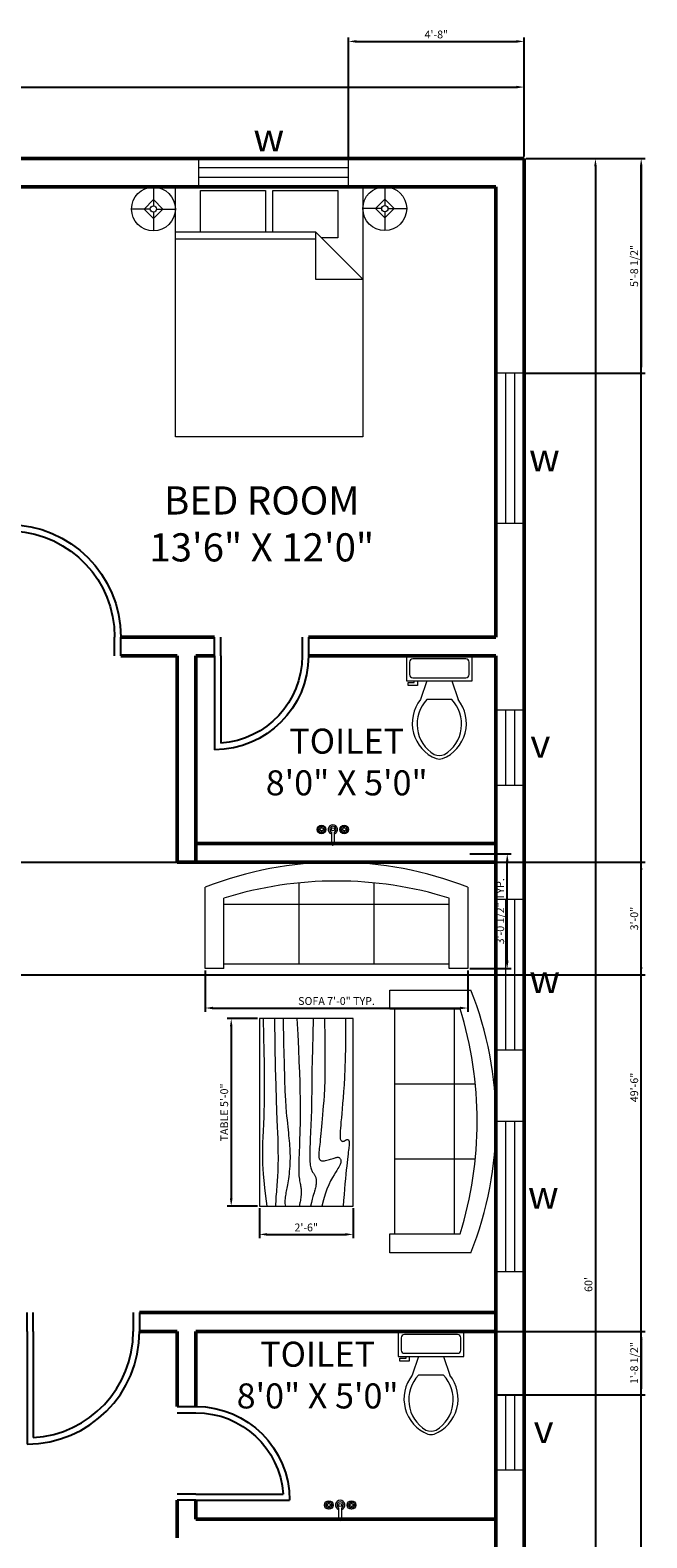
# Model space of a CAD drawing. Units: inches. Extents: x 1776 to 2338, y 1299 to 2099.
# Tile 4 of 4: x 2141 to 2338, y 1617 to 2099. Entities that reach past the tile are written whole.
import ezdxf

# ---------------------------------------------------------------- set-up
doc = ezdxf.new("R2010")
doc.units = ezdxf.units.IN
for name, color, linetype, lineweight in [('A-ANNO-DIMS', 2, 'Continuous', 18), ('A-ANNO-TEXT', 7, 'Continuous', 18), ('A-AREA-IDEN', 7, 'Continuous', 25), ('A-DOOR', 4, 'Continuous', 25), ('A-FLOR-FIXT', 9, 'Continuous', 18), ('A-FURN', 8, 'Continuous', 18), ('A-GLAZ', 4, 'Continuous', 18), ('A-WALL', 7, 'Continuous', 50), ('E-LITE', 9, 'Continuous', 18)]:
    doc.layers.add(name, color=color, linetype=linetype, lineweight=lineweight)
doc.styles.get("Standard").update_dxf_attribs({"font": 'arial.ttf'})
doc.dimstyles.new('ISO-25', dxfattribs={"dimtxt": 2.5, "dimasz": 2.5, "dimexe": 1.25, "dimexo": 0.625, "dimtad": 1, "dimdec": 0, "dimlunit": 3, "dimtxsty": 'Standard', "dimcen": 2.5, "dimadec": 0, "dimazin": 0, "dimtfac": 1, "dimtdec": 0, "dimtmove": 0, "dimatfit": 3, "dimfxl": 1, "dimarcsym": 0})

# ---------------------------------------------------------------- blocks, each defined once
blk = doc.blocks.new('Bed - Queen')
for p, q in [((0, -80.00003), (0, 0)), ((0, 0), (59.99999, 0)), ((59.99999, 0), (59.99999, -80.00003)), ((7.99999, -1.2), (28.79998, -1.2)), ((7.99999, -14.4), (7.99999, -1.2)), ((28.79998, -1.2), (28.79998, -14.4)), ((31.19999, -1.2), (51.99999, -1.2)), ((31.19999, -14.4), (31.19999, -1.2)), ((51.99999, -1.2), (51.99999, -16.4)), ((0, -14.4), (44.8, -14.4)), ((59.99999, -29.6), (44.8, -14.4)), ((44.8, -14.4), (44.8, -29.6)), ((44.8, -16.8), (0, -16.8)), ((51.99999, -16.4), (46.79936, -16.4)), ((44.8, -29.6), (59.99999, -29.6)), ((59.99999, -80.00003), (0, -80.00003))]:
    blk.add_line(p, q)
blk = doc.blocks.new('Sofa - Roundback 7 ft.')
for p, q in [((-12.00002, -32.4421), (-12.00003, -6.5971)), ((11.99997, -32.4421), (11.99998, -6.5971)), ((-36.000027, -34), (-36.000027, -11.4696)), ((-35.999844, -13.3819), (35.9998, -13.3819)), ((35.99998, -34), (35.99998, -11.4696)), ((-36.000027, -32.4421), (35.99998, -32.4421))]:
    blk.add_line(p, q)
for points in [[(-36.000027, -34), (-42.000027, -34), (-42.000027, -8)], [(41.99998, -8), (41.99998, -34), (35.99998, -34)]]:
    blk.add_lwpolyline(points)
for centre, radius, start, end in [((0, -114.25), 114.25, 68.43141, 111.5686), ((-0.00001, -127.1968), 121.1968, 72.72033, 107.2797)]:
    blk.add_arc(centre, radius, start, end)
blk = doc.blocks.new('Table - Rectangular Woodgrain 60 x 30 in.')
for p, q in [((0, 0), (0, -30)), ((60, 0), (0, 0)), ((60, -30), (60, 0)), ((0, -30), (60, -30))]:
    blk.add_line(p, q)
for points in [[(0, -2.4), (4.8155, -2.418), (9.0302, -2.4688), (12.709, -2.5477), (15.9167, -2.65), (18.7181, -2.7711), (21.1781, -2.9063), (23.3616, -3.0508), (25.3333, -3.2), (27.1477, -3.3495), (28.8172, -3.4958), (30.3437, -3.636), (31.7291, -3.7667), (32.9756, -3.8849), (34.0849, -3.9875), (35.059, -4.0714), (35.9, -4.1334), (36.6114, -4.1711), (37.2041, -4.1854), (37.6906, -4.1779), (38.0833, -4.15), (38.3948, -4.1034), (38.6375, -4.0396), (38.8239, -3.9602), (38.9666, -3.8667), (39.0764, -3.7608), (39.1573, -3.6448), (39.2116, -3.521), (39.2416, -3.3917), (39.2498, -3.2593), (39.2385, -3.1261), (39.21, -2.9944), (39.1666, -2.8667), (39.111, -2.7447), (39.0468, -2.6281), (38.978, -2.5163), (38.9083, -2.4083), (38.8418, -2.3035), (38.7823, -2.201), (38.7337, -2.1001), (38.7, -2), (38.6844, -1.9003), (38.6875, -1.8021), (38.7094, -1.707), (38.75, -1.6167), (38.8094, -1.5326), (38.8875, -1.4563), (38.9844, -1.3893), (39.1, -1.3333), (39.2351, -1.2896), (39.3937, -1.2583), (39.5804, -1.2396), (39.8, -1.2333), (40.057, -1.2396), (40.3562, -1.2583), (40.7023, -1.2896), (41.1, -1.3333), (41.5547, -1.3895), (42.0755, -1.4573), (42.6721, -1.5361), (43.3542, -1.625), (44.1316, -1.7233), (45.014, -1.8302), (46.0114, -1.9449), (47.1333, -2.0667), (48.3862, -2.1947), (49.7625, -2.3281), (51.2513, -2.4663), (52.8416, -2.6083), (54.5226, -2.7535), (56.2833, -2.9011), (58.1127, -3.0501), (60, -3.2)], [(0, -9.2), (6.5759, -9.0858), (11.9385, -9.0365), (16.2527, -9.0418), (19.6833, -9.0917), (22.3952, -9.1759), (24.5531, -9.2844), (26.322, -9.4069), (27.8666, -9.5333), (29.3241, -9.6553), (30.7203, -9.7719), (32.0532, -9.8837), (33.3208, -9.9917), (34.5213, -10.0965), (35.6526, -10.199), (36.7128, -10.2999), (37.7, -10.4), (38.6129, -10.4996), (39.4531, -10.5969), (40.223, -10.6895), (40.925, -10.775), (41.5613, -10.8512), (42.1344, -10.9156), (42.6465, -10.966), (43.1, -11), (43.4976, -11.0158), (43.8437, -11.0136), (44.143, -10.9942), (44.4, -10.9583), (44.6195, -10.9069), (44.8062, -10.8406), (44.9648, -10.7603), (45.1, -10.6667), (45.2155, -10.5598), (45.3114, -10.4365), (45.3871, -10.2929), (45.4416, -10.125), (45.4743, -9.929), (45.4844, -9.7011), (45.4709, -9.4371), (45.4333, -9.1333), (45.3716, -8.7883), (45.2896, -8.4104), (45.1919, -8.0107), (45.0833, -7.6), (44.9685, -7.1893), (44.8521, -6.7896), (44.7388, -6.4117), (44.6333, -6.0667), (44.54, -5.7628), (44.4614, -5.4979), (44.4001, -5.2675), (44.3583, -5.0667), (44.3384, -4.8909), (44.3427, -4.7354), (44.3736, -4.5956), (44.4333, -4.4667), (44.5236, -4.3453), (44.6427, -4.2333), (44.7884, -4.1339), (44.9583, -4.05), (45.1501, -3.9849), (45.3614, -3.9417), (45.59, -3.9234), (45.8333, -3.9333), (46.0915, -3.9749), (46.3734, -4.0531), (46.6906, -4.1736), (47.0542, -4.3417), (47.4756, -4.5629), (47.9661, -4.8427), (48.5372, -5.1866), (49.2, -5.6), (49.9676, -6.0844), (50.8594, -6.625), (51.8965, -7.2031), (53.1, -7.8), (54.491, -8.3969), (56.0906, -8.975), (57.9199, -9.5156), (60, -10)], [(0, -12.8), (5.1847, -12.9322), (9.6213, -13.0323), (13.3963, -13.1059), (16.5958, -13.1583), (19.3063, -13.1952), (21.614, -13.2219), (23.6054, -13.2439), (25.3666, -13.2667), (26.9728, -13.2947), (28.4531, -13.3281), (29.8256, -13.3663), (31.1083, -13.4083), (32.3191, -13.4535), (33.476, -13.501), (34.597, -13.5501), (35.7, -13.6), (36.7984, -13.6497), (37.8875, -13.6979), (38.9578, -13.743), (40, -13.7833), (41.0047, -13.8174), (41.9625, -13.8438), (42.864, -13.8607), (43.7, -13.8667), (44.4631, -13.8604), (45.1552, -13.8417), (45.7801, -13.8104), (46.3416, -13.7667), (46.8439, -13.7104), (47.2906, -13.6417), (47.6858, -13.5604), (48.0333, -13.4667), (48.3375, -13.3608), (48.6042, -13.2448), (48.8396, -13.121), (49.05, -12.9917), (49.2417, -12.8593), (49.4208, -12.7261), (49.5937, -12.5944), (49.7667, -12.4667), (49.9452, -12.3451), (50.1323, -12.2313), (50.3303, -12.1268), (50.5416, -12.0333), (50.7686, -11.9524), (51.0135, -11.8854), (51.2788, -11.8341), (51.5666, -11.8), (51.8785, -11.7843), (52.2116, -11.7865), (52.562, -11.8059), (52.926, -11.8417), (53.2998, -11.8931), (53.6795, -11.9594), (54.0614, -12.0397), (54.4416, -12.1333), (54.8223, -12.2401), (55.2293, -12.3625), (55.6942, -12.5037), (56.2489, -12.6667), (56.9251, -12.8547), (57.7545, -13.0708), (58.7689, -13.3182), (60, -13.6)], [(0, -18), (5.124, -17.7273), (9.6609, -17.5057), (13.6705, -17.3303), (17.2125, -17.1958), (20.3467, -17.0973), (23.1328, -17.0297), (25.6307, -16.9878), (27.9, -16.9667), (29.9928, -16.9617), (31.9302, -16.9703), (33.7254, -16.9907), (35.3917, -17.0208), (36.9423, -17.0588), (38.3906, -17.1026), (39.7499, -17.1503), (41.0333, -17.2), (42.2519, -17.2496), (43.4073, -17.2969), (44.4986, -17.3395), (45.525, -17.375), (46.4858, -17.4012), (47.3802, -17.4156), (48.2074, -17.416), (48.9667, -17.4), (49.6583, -17.3662), (50.2872, -17.3167), (50.8595, -17.2547), (51.3812, -17.1833), (51.8584, -17.1057), (52.2971, -17.025), (52.7034, -16.9443), (53.0833, -16.8667), (53.443, -16.7951), (53.789, -16.7313), (54.128, -16.6768), (54.4666, -16.6334), (54.8115, -16.6024), (55.1693, -16.5854), (55.5465, -16.5841), (55.95, -16.6), (56.3828, -16.6337), (56.8346, -16.6823), (57.2915, -16.7418), (57.7396, -16.8084), (58.165, -16.878), (58.5539, -16.9469), (58.8924, -17.0111), (59.1666, -17.0667), (59.3679, -17.1107), (59.5078, -17.1438), (59.6032, -17.1675), (59.6708, -17.1833), (59.7275, -17.193), (59.7901, -17.1979), (59.8753, -17.1998), (60, -17.2)], [(0, -22.4), (8.0098, -22.2501), (14.4094, -22.1011), (19.4168, -21.9535), (23.25, -21.8083), (26.1269, -21.6663), (28.2656, -21.5281), (29.884, -21.3947), (31.2, -21.2667), (32.3967, -21.1448), (33.5172, -21.0292), (34.5697, -20.9198), (35.5625, -20.8167), (36.5037, -20.7198), (37.4015, -20.6292), (38.2642, -20.5448), (39.1, -20.4667), (39.9164, -20.3951), (40.7187, -20.3313), (41.5117, -20.2768), (42.3, -20.2333), (43.0883, -20.2024), (43.8812, -20.1854), (44.6836, -20.1841), (45.5, -20.2), (46.3328, -20.234), (47.1747, -20.2844), (48.0163, -20.3488), (48.8479, -20.425), (49.66, -20.5106), (50.4429, -20.6031), (51.1872, -20.7004), (51.8833, -20.8), (52.5246, -20.8999), (53.1166, -20.9995), (53.6681, -21.0983), (54.1875, -21.1958), (54.6834, -21.2919), (55.1646, -21.3859), (55.6394, -21.4777), (56.1167, -21.5667), (56.6028, -21.6515), (57.0961, -21.7266), (57.5929, -21.7852), (58.0896, -21.8208), (58.5823, -21.8268), (59.0674, -21.7964), (59.5412, -21.723), (60, -21.6)], [(0, -25.2), (8.6355, -25.0504), (15.7026, -24.9031), (21.4049, -24.7606), (25.9458, -24.625), (29.529, -24.4988), (32.3578, -24.3844), (34.6359, -24.284), (36.5667, -24.2), (38.3213, -24.1341), (39.9417, -24.0854), (41.437, -24.0523), (42.8167, -24.0333), (44.0901, -24.0268), (45.2667, -24.0313), (46.3557, -24.0451), (47.3667, -24.0667), (48.309, -24.0947), (49.1928, -24.1287), (50.0284, -24.168), (50.826, -24.2125), (51.5959, -24.2617), (52.3483, -24.3151), (53.0935, -24.3725), (53.8417, -24.4334), (54.6009, -24.497), (55.3699, -24.561), (56.1454, -24.6226), (56.9239, -24.6792), (57.7021, -24.7279), (58.4764, -24.7662), (59.2435, -24.7911), (60, -24.8)], [(0, -28.8), (5.6867, -28.6681), (10.45, -28.5698), (14.407, -28.5012), (17.675, -28.4584), (20.3711, -28.4374), (22.6125, -28.4344), (24.5164, -28.4455), (26.2, -28.4667), (27.762, -28.4947), (29.2276, -28.5281), (30.6033, -28.5663), (31.8958, -28.6084), (33.1118, -28.6535), (34.2578, -28.7011), (35.3405, -28.7501), (36.3666, -28.8), (37.3443, -28.8497), (38.288, -28.8974), (39.2137, -28.9412), (40.1375, -28.9792), (41.0753, -29.0093), (42.0432, -29.0297), (43.0572, -29.0384), (44.1333, -29.0333), (45.2936, -29.0114), (46.5843, -28.9641), (48.0579, -28.8816), (49.7666, -28.7542), (51.7629, -28.5721), (54.0989, -28.3255), (56.8272, -28.0048), (60, -27.6)]]:
    blk.add_lwpolyline(points)
blk = doc.blocks.new('Lamp - Table')
for p, q in [((0, 7), (0, 1)), ((-1, 0), (-7, 0)), ((0, 3), (-3, 0)), ((-3, 0), (0, -3)), ((3, 0), (0, 3)), ((0, -3), (3, 0)), ((1, 0), (7, 0)), ((0, -1), (0, -7))]:
    blk.add_line(p, q)
for radius in [7, 1]:
    blk.add_circle((0, 0), radius)
blk = doc.blocks.new('Toilet - top')
for p, q in [((9.5, -6), (9.5, -2)), ((-10, -8.5), (-8, -8.5)), ((-10, -9.5), (-10, -8.5)), ((-7, -9.5), (-10, -9.5)), ((-8, -8.5), (-8, -8)), ((-7, -8), (-7, -9.5)), ((-4, -8), (-6, -14)), ((4, -8), (6, -14)), ((4, -14), (-4, -14))]:
    blk.add_line(p, q)
blk.add_lwpolyline([(10.5, -8), (10.5, 0), (-10.5, 0), (-10.5, -8)], close=True)
for points in [[(-9.5, -2), (-9.5, -6)], [(8.5, -1), (-8.5, -1)], [(-8.5, -7), (8.5, -7)]]:
    blk.add_lwpolyline(points)
for centre, radius, start, end in [((-8.62, -1.88), 0.884, 81.8699, 188.1301), ((8.62, -1.88), 0.884, 351.8699, 98.1301), ((-8.62, -6.12), 0.884, 171.8699, 278.1301), ((8.62, -6.12), 0.884, 261.8699, 8.1301), ((3.52, -21.58), 12.17, 141.4691, 247.9714), ((4.2, -21.82), 11.33, 136.3677, 238.9468), ((-3.52, -21.58), 12.17, 292.0284, 38.5307), ((-4.2, -21.82), 11.33, 301.053, 43.6321), ((0, -27.88), 4, 245.7318, 294.2682), ((0, -29), 4, 254.8605, 285.1395)]:
    blk.add_arc(centre, radius, start, end)
blk = doc.blocks.new('Faucet - Bathroom top')
for p, q in [((-4.107, 0.125), (-4.375, 0.125)), ((-3.75, 0.4788), (-3.75, 0.75)), ((-3.5, 0.482), (-3.5, 0.75)), ((-3.1461, 0.125), (-2.875, 0.125)), ((3.143, 0.125), (2.875, 0.125)), ((3.5, 0.4788), (3.5, 0.75)), ((3.75, 0.482), (3.75, 0.75)), ((4.1039, 0.125), (4.375, 0.125)), ((-4.1039, -0.125), (-4.375, -0.125)), ((-3.75, -0.4821), (-3.75, -0.75)), ((-3.5, -0.4789), (-3.5, -0.75)), ((-3.143, -0.125), (-2.875, -0.125)), ((-0.5, -0.8639), (-0.5, -4.5)), ((0.5, -4.5), (0.5, -0.8631)), ((3.1461, -0.125), (2.875, -0.125)), ((3.5, -0.4821), (3.5, -0.75)), ((3.75, -0.4789), (3.75, -0.75)), ((4.107, -0.125), (4.375, -0.125))]:
    blk.add_line(p, q)
for centre, radius in [((-3.625, 0), 1.375), ((-4.625, 0), 0.2795), ((-3.625, 0), 0.5), ((-3.625, 1), 0.2795), ((-2.625, 0), 0.2795), ((0, 0), 0.5), ((3.625, 0), 1.375), ((2.625, 0), 0.2795), ((3.625, 0), 0.5), ((3.625, 1), 0.2795), ((4.625, 0), 0.2795), ((-3.625, -1), 0.2795), ((3.625, -1), 0.2795)]:
    blk.add_circle(centre, radius)
for centre, radius, start, end in [((-3.625, 0), 1, 105.2407, 164.2093), ((-3.625, 0), 1, 16.44125, 74.07887), ((0, 0), 1.5, 289.6514, 250.3603), ((0, 0), 1, 300.3431, 239.7554), ((3.625, 0), 1, 106.12, 164.0884), ((3.625, 0), 1, 16.23422, 73.90469), ((-3.625, 0), 1, 196.2342, 253.9047), ((-3.625, 0), 1, 286.12, 344.0884), ((0, -4.5), 0.5, 180, 0), ((3.625, 0), 1, 196.4413, 254.0789), ((3.625, 0), 1, 285.2407, 344.2093)]:
    blk.add_arc(centre, radius, start, end)
blk = doc.blocks.new('*D12')
at = {"layer": 'A-ANNO-DIMS', "color": 0, "lineweight": -2, "transparency": 16777216}
for p, q in [((1818.74, 2058.84), (1818.74, 2082.32)), ((1821.24, 2081.07), (2296.24, 2081.07)), ((2298.74, 2058.84), (2298.74, 2082.32))]:
    blk.add_line(p, q, dxfattribs=at)
at = {"layer": 'A-ANNO-DIMS', "color": 0, "transparency": 16777216}
for points in [[(1821.24, 2081.49), (1821.24, 2080.65), (1818.74, 2081.07)], [(2296.24, 2081.49), (2296.24, 2080.65), (2298.74, 2081.07)]]:
    blk.add_solid(points, dxfattribs=at)
at = {"layer": 'Defpoints', "color": 0, "transparency": 16777216}
for p in [(2298.74, 2081.07), (1818.74, 2058.22), (2298.74, 2058.22)]:
    blk.add_point(p, dxfattribs=at)
at = {"layer": 'A-ANNO-DIMS', "color": 0, "transparency": 16777216, "insert": (2058.74, 2082.97), "char_height": 2.5, "attachment_point": 5}
blk.add_mtext("40'", dxfattribs=at)
blk = doc.blocks.new('*D13')
at = {"layer": 'A-ANNO-DIMS', "color": 0, "lineweight": -2, "transparency": 16777216}
for p, q in [((2299.36, 2058.22), (2322.8, 2058.22)), ((2321.55, 2055.72), (2321.55, 1340.72)), ((2299.36, 1338.22), (2322.8, 1338.22))]:
    blk.add_line(p, q, dxfattribs=at)
at = {"layer": 'A-ANNO-DIMS', "color": 0, "transparency": 16777216}
for points in [[(2321.14, 2055.72), (2321.97, 2055.72), (2321.55, 2058.22)], [(2321.14, 1340.72), (2321.97, 1340.72), (2321.55, 1338.22)]]:
    blk.add_solid(points, dxfattribs=at)
at = {"layer": 'Defpoints', "color": 0, "transparency": 16777216}
for p in [(2298.74, 2058.22), (2298.74, 1338.22), (2321.55, 1338.22)]:
    blk.add_point(p, dxfattribs=at)
at = {"layer": 'A-ANNO-DIMS', "color": 0, "transparency": 16777216, "insert": (2319.65, 1698.22), "char_height": 2.5, "attachment_point": 5, "rotation": 90}
blk.add_mtext("60'", dxfattribs=at)
blk = doc.blocks.new('WIN-48IN')
for p, q in [((48, 9), (0, 9)), ((0, 9), (0, 0)), ((48, 6), (0, 6)), ((48, 0), (48, 9)), ((0, 3), (48, 3)), ((0, 0), (48, 0))]:
    blk.add_line(p, q)
blk = doc.blocks.new('VENT-24IN')
for p, q in [((9, 24), (0, 24)), ((0, 24), (0, 0)), ((3, 24), (3, 0)), ((6, 0), (6, 24)), ((9, 0), (9, 24)), ((0, 0), (9, 0))]:
    blk.add_line(p, q)
blk = doc.blocks.new('DOOR-36IN')
for p, q in [((34, 6), (34, 39.94)), ((36, 6), (36, 42)), ((0, 0), (0, 6)), ((2, 0), (2, 6)), ((34, 6), (34, 0)), ((36, 6), (36, 0))]:
    blk.add_line(p, q)
for radius, start in [(36, 90), (34, 93.3723)]:
    blk.add_arc((36, 6), radius, start, 180)
blk = doc.blocks.new('DOOR-30IN')
for p, q in [((0, 36), (0, 30)), ((2, 36), (2, 30)), ((28, 30), (28, 36)), ((30, 30), (30, 36)), ((28, 30), (28, 2.07)), ((30, 30), (30, 0))]:
    blk.add_line(p, q)
for radius, end in [(30, 270), (28, 265.904)]:
    blk.add_arc((30, 30), radius, 180, end)
blk = doc.blocks.new('*D34')
at = {"layer": 'A-ANNO-DIMS', "color": 0, "lineweight": -2, "transparency": 16777216}
for p, q in [((2196.74, 1798.59), (2196.74, 1785.37)), ((2280.74, 1798.59), (2280.74, 1785.37)), ((2199.24, 1786.62), (2278.24, 1786.62))]:
    blk.add_line(p, q, dxfattribs=at)
at = {"layer": 'A-ANNO-DIMS', "color": 0, "transparency": 16777216}
for points in [[(2199.24, 1787.04), (2199.24, 1786.2), (2196.74, 1786.62)], [(2278.24, 1787.04), (2278.24, 1786.2), (2280.74, 1786.62)]]:
    blk.add_solid(points, dxfattribs=at)
at = {"layer": 'Defpoints', "color": 0, "transparency": 16777216}
for p in [(2196.74, 1799.22), (2280.74, 1799.22), (2280.74, 1786.62)]:
    blk.add_point(p, dxfattribs=at)
at = {"layer": 'A-ANNO-DIMS', "color": 0, "transparency": 16777216, "insert": (2238.74, 1788.54), "char_height": 2.5, "attachment_point": 5}
blk.add_mtext('SOFA 7\'-0" TYP.', dxfattribs=at)
blk = doc.blocks.new('*D35')
at = {"layer": 'A-ANNO-DIMS', "color": 0, "lineweight": -2, "transparency": 16777216}
for p, q in [((2281.36, 1835.89), (2294.59, 1835.89)), ((2293.34, 1801.72), (2293.34, 1833.39)), ((2281.36, 1799.22), (2294.59, 1799.22))]:
    blk.add_line(p, q, dxfattribs=at)
at = {"layer": 'A-ANNO-DIMS', "color": 0, "transparency": 16777216}
for points in [[(2292.92, 1833.39), (2293.76, 1833.39), (2293.34, 1835.89)], [(2292.92, 1801.72), (2293.76, 1801.72), (2293.34, 1799.22)]]:
    blk.add_solid(points, dxfattribs=at)
at = {"layer": 'Defpoints', "color": 0, "transparency": 16777216}
for p in [(2280.74, 1835.89), (2293.34, 1835.89), (2280.74, 1799.22)]:
    blk.add_point(p, dxfattribs=at)
at = {"layer": 'A-ANNO-DIMS', "color": 0, "transparency": 16777216, "insert": (2291.42, 1817.55), "char_height": 2.5, "attachment_point": 5, "rotation": 90}
blk.add_mtext('3\'-0 1/2" TYP.', dxfattribs=at)
blk = doc.blocks.new('*D36')
at = {"layer": 'A-ANNO-DIMS', "color": 0, "lineweight": -2, "transparency": 16777216}
for p, q in [((2213.43, 1783.24), (2203.8, 1783.24)), ((2205.05, 1780.74), (2205.05, 1725.74)), ((2213.43, 1723.24), (2203.8, 1723.24))]:
    blk.add_line(p, q, dxfattribs=at)
at = {"layer": 'A-ANNO-DIMS', "color": 0, "transparency": 16777216}
for points in [[(2204.64, 1780.74), (2205.47, 1780.74), (2205.05, 1783.24)], [(2204.64, 1725.74), (2205.47, 1725.74), (2205.05, 1723.24)]]:
    blk.add_solid(points, dxfattribs=at)
at = {"layer": 'Defpoints', "color": 0, "transparency": 16777216}
for p in [(2214.05, 1783.24), (2205.05, 1723.24), (2214.05, 1723.24)]:
    blk.add_point(p, dxfattribs=at)
at = {"layer": 'A-ANNO-DIMS', "color": 0, "transparency": 16777216, "insert": (2203.15, 1753.24), "char_height": 2.5, "attachment_point": 5, "rotation": 90}
blk.add_mtext('TABLE 5\'-0"', dxfattribs=at)
blk = doc.blocks.new('*D37')
at = {"layer": 'A-ANNO-DIMS', "color": 0, "lineweight": -2, "transparency": 16777216}
for p, q in [((2214.05, 1722.61), (2214.05, 1712.99)), ((2244.05, 1722.61), (2244.05, 1712.99)), ((2216.55, 1714.24), (2241.55, 1714.24))]:
    blk.add_line(p, q, dxfattribs=at)
at = {"layer": 'A-ANNO-DIMS', "color": 0, "transparency": 16777216}
for points in [[(2216.55, 1714.66), (2216.55, 1713.82), (2214.05, 1714.24)], [(2241.55, 1714.66), (2241.55, 1713.82), (2244.05, 1714.24)]]:
    blk.add_solid(points, dxfattribs=at)
at = {"layer": 'Defpoints', "color": 0, "transparency": 16777216}
for p in [(2214.05, 1723.24), (2244.05, 1723.24), (2244.05, 1714.24)]:
    blk.add_point(p, dxfattribs=at)
at = {"layer": 'A-ANNO-DIMS', "color": 0, "transparency": 16777216, "insert": (2229.05, 1716.14), "char_height": 2.5, "attachment_point": 5}
blk.add_mtext('2\'-6"', dxfattribs=at)
blk = doc.blocks.new('*D42')
at = {"layer": 'A-ANNO-DIMS', "color": 0, "lineweight": -2, "transparency": 16777216}
for p, q in [((2299.36, 2058.22), (2337.44, 2058.22)), ((2336.19, 1466.72), (2336.19, 2055.72)), ((2290.36, 1464.22), (2337.44, 1464.22))]:
    blk.add_line(p, q, dxfattribs=at)
at = {"layer": 'A-ANNO-DIMS', "color": 0, "transparency": 16777216}
for points in [[(2335.77, 2055.72), (2336.61, 2055.72), (2336.19, 2058.22)], [(2335.77, 1466.72), (2336.61, 1466.72), (2336.19, 1464.22)]]:
    blk.add_solid(points, dxfattribs=at)
at = {"layer": 'Defpoints', "color": 0, "transparency": 16777216}
for p in [(2298.74, 2058.22), (2336.19, 2058.22), (2289.74, 1464.22)]:
    blk.add_point(p, dxfattribs=at)
at = {"layer": 'A-ANNO-DIMS', "color": 0, "transparency": 16777216, "insert": (2334.29, 1761.22), "char_height": 2.5, "attachment_point": 5, "rotation": 90}
blk.add_mtext('49\'-6"', dxfattribs=at)
blk = doc.blocks.new('*D48')
at = {"layer": 'A-ANNO-DIMS', "color": 0, "lineweight": -2, "transparency": 16777216}
for p, q in [((1936.36, 1833.22), (2337.44, 1833.22)), ((2336.19, 1799.72), (2336.19, 1830.72)), ((1936.36, 1797.22), (2337.44, 1797.22))]:
    blk.add_line(p, q, dxfattribs=at)
at = {"layer": 'A-ANNO-DIMS', "color": 0, "transparency": 16777216}
for points in [[(2335.77, 1830.72), (2336.61, 1830.72), (2336.19, 1833.22)], [(2335.77, 1799.72), (2336.61, 1799.72), (2336.19, 1797.22)]]:
    blk.add_solid(points, dxfattribs=at)
at = {"layer": 'Defpoints', "color": 0, "transparency": 16777216}
for p in [(1935.74, 1833.22), (2336.19, 1833.22), (1935.74, 1797.22)]:
    blk.add_point(p, dxfattribs=at)
at = {"layer": 'A-ANNO-DIMS', "color": 0, "transparency": 16777216, "insert": (2334.29, 1815.22), "char_height": 2.5, "attachment_point": 5, "rotation": 90}
blk.add_mtext('3\'-0"', dxfattribs=at)
blk = doc.blocks.new('*D52')
at = {"layer": 'A-ANNO-DIMS', "color": 0, "lineweight": -2, "transparency": 16777216}
for p, q in [((2242.6, 2058.84), (2242.6, 2096.92)), ((2245.1, 2095.67), (2296.24, 2095.67)), ((2298.74, 2058.84), (2298.74, 2096.92))]:
    blk.add_line(p, q, dxfattribs=at)
at = {"layer": 'A-ANNO-DIMS', "color": 0, "transparency": 16777216}
for points in [[(2245.1, 2096.09), (2245.1, 2095.25), (2242.6, 2095.67)], [(2296.24, 2096.09), (2296.24, 2095.25), (2298.74, 2095.67)]]:
    blk.add_solid(points, dxfattribs=at)
at = {"layer": 'Defpoints', "color": 0, "transparency": 16777216}
for p in [(2298.74, 2095.67), (2242.6, 2058.22), (2298.74, 2058.22)]:
    blk.add_point(p, dxfattribs=at)
at = {"layer": 'A-ANNO-DIMS', "color": 0, "transparency": 16777216, "insert": (2270.67, 2097.57), "char_height": 2.5, "attachment_point": 5}
blk.add_mtext('4\'-8"', dxfattribs=at)
blk = doc.blocks.new('*D54')
at = {"layer": 'A-ANNO-DIMS', "color": 0, "lineweight": -2, "transparency": 16777216}
for p, q in [((2299.36, 2058.22), (2337.44, 2058.22)), ((2336.19, 2055.72), (2336.19, 1992.09)), ((2299.36, 1989.59), (2337.44, 1989.59))]:
    blk.add_line(p, q, dxfattribs=at)
at = {"layer": 'A-ANNO-DIMS', "color": 0, "transparency": 16777216}
for points in [[(2335.77, 2055.72), (2336.61, 2055.72), (2336.19, 2058.22)], [(2335.77, 1992.09), (2336.61, 1992.09), (2336.19, 1989.59)]]:
    blk.add_solid(points, dxfattribs=at)
at = {"layer": 'Defpoints', "color": 0, "transparency": 16777216}
for p in [(2298.74, 2058.22), (2298.74, 1989.59), (2336.19, 1989.59)]:
    blk.add_point(p, dxfattribs=at)
at = {"layer": 'A-ANNO-DIMS', "color": 0, "transparency": 16777216, "insert": (2334.27, 2023.9), "char_height": 2.5, "attachment_point": 5, "rotation": 90}
blk.add_mtext('5\'-8 1/2"', dxfattribs=at)
blk = doc.blocks.new('*D57')
at = {"layer": 'A-ANNO-DIMS', "color": 0, "lineweight": -2, "transparency": 16777216}
for p, q in [((2290.36, 1683.22), (2337.44, 1683.22)), ((2336.19, 1680.72), (2336.19, 1665.46)), ((2290.36, 1662.96), (2337.44, 1662.96))]:
    blk.add_line(p, q, dxfattribs=at)
at = {"layer": 'A-ANNO-DIMS', "color": 0, "transparency": 16777216}
for points in [[(2335.77, 1680.72), (2336.61, 1680.72), (2336.19, 1683.22)], [(2335.77, 1665.46), (2336.61, 1665.46), (2336.19, 1662.96)]]:
    blk.add_solid(points, dxfattribs=at)
at = {"layer": 'Defpoints', "color": 0, "transparency": 16777216}
for p in [(2289.74, 1683.22), (2289.74, 1662.96), (2336.19, 1662.96)]:
    blk.add_point(p, dxfattribs=at)
at = {"layer": 'A-ANNO-DIMS', "color": 0, "transparency": 16777216, "insert": (2334.27, 1673.09), "char_height": 2.5, "attachment_point": 5, "rotation": 90}
blk.add_mtext('1\'-8 1/2"', dxfattribs=at)

msp = doc.modelspace()

# ---------------------------------------------------------------- linework, layer by layer
at = {"layer": 'A-DOOR'}
msp.add_line((2141.74, 1647.27), (2141.74, 1647.22), dxfattribs=at)
at = {"layer": 'A-WALL'}
for p, q in [((1818.74, 2058.22), (2298.74, 2058.22)), ((2298.74, 2058.22), (2298.74, 1338.22)), ((2127.74, 2049.22), (2289.74, 2049.22)), ((2289.74, 2049.22), (2289.74, 1905.22)), ((2169.74, 1905.22), (2199.74, 1905.22)), ((2229.74, 1905.22), (2289.74, 1905.22)), ((2169.74, 1899.22), (2187.74, 1899.22)), ((2187.74, 1899.22), (2187.74, 1833.22)), ((2187.74, 1899.22), (2187.74, 1833.22)), ((2193.74, 1899.22), (2193.74, 1839.22)), ((2193.74, 1899.22), (2199.74, 1899.22)), ((2193.74, 1899.22), (2193.74, 1833.22)), ((2193.74, 1899.22), (2199.74, 1899.22)), ((2229.74, 1899.22), (2289.74, 1899.22)), ((2289.74, 1899.22), (2289.74, 1473.22)), ((2193.74, 1839.22), (2289.74, 1839.22)), ((2187.74, 1833.22), (2289.74, 1833.22)), ((2175.74, 1689.22), (2187.74, 1689.22)), ((2187.74, 1689.22), (2289.74, 1689.22)), ((2175.74, 1683.22), (2187.74, 1683.22)), ((2187.74, 1683.22), (2187.74, 1659.22)), ((2193.74, 1683.22), (2289.74, 1683.22)), ((2193.74, 1683.22), (2193.74, 1659.22)), ((2187.74, 1629.22), (2187.74, 1617.22)), ((2193.74, 1623.22), (2193.74, 1629.22)), ((2193.74, 1629.22), (2193.74, 1623.22)), ((2193.74, 1623.22), (2289.74, 1623.22))]:
    msp.add_line(p, q, dxfattribs=at)

# ---------------------------------------------------------------- block references
at = {"layer": 'A-DOOR', "extrusion": (0, 0, -1), "zscale": -1}
for name, p in [('DOOR-36IN', (-2169.74, 1899.22)), ('DOOR-30IN', (-2229.74, 1869.22))]:
    msp.add_blockref(name, p, dxfattribs=at)
at = {"layer": 'A-DOOR', "rotation": 180}
msp.add_blockref('DOOR-36IN', (2175.74, 1689.22), dxfattribs=at)
at = {"layer": 'A-DOOR', "extrusion": (0, 0, -1), "zscale": -1, "rotation": 269.9999999999998}
msp.add_blockref('DOOR-30IN', (-2223.74, 1659.22), dxfattribs=at)
at = {"layer": 'A-FLOR-FIXT'}
for name, p in [('Toilet - top', (2271.62, 1899.22)), ('Faucet - Bathroom top', (2237.59, 1843.72)), ('Toilet - top', (2268.96, 1683.22)), ('Faucet - Bathroom top', (2239.92, 1627.72))]:
    msp.add_blockref(name, p, dxfattribs=at)
at = {"layer": 'A-FURN'}
for name, p in [('Bed - Queen', (2187.18, 2049.22)), ('Sofa - Roundback 7 ft.', (2238.74, 1833.22))]:
    msp.add_blockref(name, p, dxfattribs=at)
at = {"layer": 'A-FURN', "rotation": 270}
for name, p in [('Sofa - Roundback 7 ft.', (2289.74, 1750.38)), ('Table - Rectangular Woodgrain 60 x 30 in.', (2244.05, 1783.24))]:
    msp.add_blockref(name, p, dxfattribs=at)
at = {"layer": 'A-GLAZ'}
for name, p in [('WIN-48IN', (2194.59, 2049.22)), ('VENT-24IN', (2289.74, 1857.87)), ('VENT-24IN', (2289.74, 1638.96))]:
    msp.add_blockref(name, p, dxfattribs=at)
for p, rotation in [((2289.74, 1989.59), 269.9999999999969), ((2289.74, 1821.28), 269.999999999997), ((2289.74, 1750.38), 269.9999999999973)]:
    msp.add_blockref('WIN-48IN', p, dxfattribs=dict(at, rotation=rotation))
at = {"layer": 'E-LITE'}
for p in [(2180.18, 2042.08), (2254.18, 2042.23)]:
    msp.add_blockref('Lamp - Table', p, dxfattribs=at)

# ---------------------------------------------------------------- texts
at = {"layer": 'A-ANNO-TEXT', "char_height": 9, "attachment_point": 1}
for s, heights, insert in [('\\pxqc;w', [0], (2191.96, 2069.49)), ('\\pxqc;w', [0], (2280.11, 1967.18)), ('\\pxqc;v', [47.58], (2278.82, 1875.66)), ('\\pxqc;w', [0], (2280.2, 1800.38)), ('\\pxqc;w', [0], (2279.76, 1731.44)), ('\\pxqc;v', [47.58], (2279.86, 1656.52))]:
    msp.add_mtext_dynamic_manual_height_columns(s, width=50.2204, gutter_width=12.5, heights=heights, dxfattribs=dict(at, insert=insert))
at = {"layer": 'A-AREA-IDEN', "attachment_point": 1}
for s, width, insert, char_height in [('\\pxqc;BED ROOM \\P13\'6" X 12\'0"', 105.4264, (2162.11, 1953.41), 9), ('\\pxqc;TOILET\\P8\'0" X 5\'0"', 54.6133, (2214.69, 1875.95), 8), ('\\pxqc;TOILET\\P8\'0" X 5\'0"', 54.6133, (2205.38, 1679.93), 8)]:
    msp.add_mtext_dynamic_manual_height_columns(s, width=width, gutter_width=12.5, heights=[0], dxfattribs=dict(at, insert=insert, char_height=char_height))

# ---------------------------------------------------------------- dimensions: what is measured, and where the dimension line sits
at = {"layer": 'A-ANNO-DIMS'}
for base, p1, p2, override, picture, middle in [((2298.74, 2095.67), (2242.6, 2058.22), (2298.74, 2058.22), {"dimdec": 1, "dimlfac": 1, "dimrnd": 0, "dimzin": 1, "dimdsep": 46, "dimlunit": 4, "dimfrac": 2}, '*D52', (2270.67, 2097.57)), ((2298.74, 2081.07), (1818.74, 2058.22), (2298.74, 2058.22), {"dimclrd": 0, "dimclre": 0, "dimclrt": 0}, '*D12', (2058.74, 2082.97)), ((2244.05, 1714.24), (2214.05, 1723.24), (2244.05, 1723.24), {"dimdec": 1, "dimlfac": 1, "dimrnd": 0, "dimzin": 1, "dimdsep": 46, "dimlunit": 4, "dimfrac": 2}, '*D37', (2229.05, 1716.14))]:
    dim = msp.add_linear_dim(base=base, p1=p1, p2=p2, dimstyle='ISO-25', override=override, dxfattribs=at)
    dim.commit()
    dim.dimension.update_dxf_attribs({"geometry": picture, "text_midpoint": middle})
for base, p1, p2, override, picture, middle in [((2336.19, 2058.22), (2289.74, 1464.22), (2298.74, 2058.22), {"dimdec": 1, "dimlfac": 1, "dimrnd": 0, "dimzin": 1, "dimdsep": 46, "dimlunit": 4, "dimfrac": 2}, '*D42', (2334.29, 1761.22)), ((2321.55, 1338.22), (2298.74, 2058.22), (2298.74, 1338.22), {"dimclrd": 0, "dimclre": 0, "dimclrt": 0}, '*D13', (2319.65, 1698.22)), ((2336.19, 1989.59), (2298.74, 2058.22), (2298.74, 1989.59), {"dimdec": 1, "dimlfac": 1, "dimrnd": 0, "dimzin": 1, "dimdsep": 46, "dimlunit": 4, "dimfrac": 2}, '*D54', (2334.27, 2023.9)), ((2336.19, 1833.22), (1935.74, 1797.22), (1935.74, 1833.22), {"dimdec": 1, "dimlfac": 1, "dimrnd": 0, "dimzin": 1, "dimdsep": 46, "dimlunit": 4, "dimfrac": 2}, '*D48', (2334.29, 1815.22)), ((2336.19, 1662.96), (2289.74, 1683.22), (2289.74, 1662.96), {"dimdec": 1, "dimlfac": 1, "dimrnd": 0, "dimzin": 1, "dimdsep": 46, "dimlunit": 4, "dimfrac": 2}, '*D57', (2334.27, 1673.09))]:
    dim = msp.add_linear_dim(base=base, p1=p1, p2=p2, angle=90, dimstyle='ISO-25', override=override, dxfattribs=at)
    dim.commit()
    dim.dimension.update_dxf_attribs({"geometry": picture, "text_midpoint": middle})
for base, p1, p2, angle, text, picture, middle in [((2293.34, 1835.89), (2280.74, 1799.22), (2280.74, 1835.89), 90, '<> TYP.', '*D35', (2291.42, 1817.55)), ((2205.05, 1723.24), (2214.05, 1783.24), (2214.05, 1723.24), 270, 'TABLE <>', '*D36', (2203.15, 1753.24))]:
    dim = msp.add_linear_dim(base=base, p1=p1, p2=p2, angle=angle, text=text, dimstyle='ISO-25', override={"dimdec": 1, "dimlfac": 1, "dimrnd": 0, "dimzin": 1, "dimdsep": 46, "dimlunit": 4, "dimfrac": 2}, dxfattribs=at)
    dim.commit()
    dim.dimension.update_dxf_attribs({"geometry": picture, "text_midpoint": middle})
dim = msp.add_linear_dim(base=(2280.74, 1786.62), p1=(2196.74, 1799.22), p2=(2280.74, 1799.22), text='SOFA <> TYP.', dimstyle='ISO-25', override={"dimdec": 1, "dimlfac": 1, "dimrnd": 0, "dimzin": 1, "dimdsep": 46, "dimlunit": 4, "dimfrac": 2}, dxfattribs=at)
dim.commit()
dim.dimension.update_dxf_attribs({"geometry": '*D34', "text_midpoint": (2238.74, 1788.54)})

doc.saveas('drawing.dxf')
